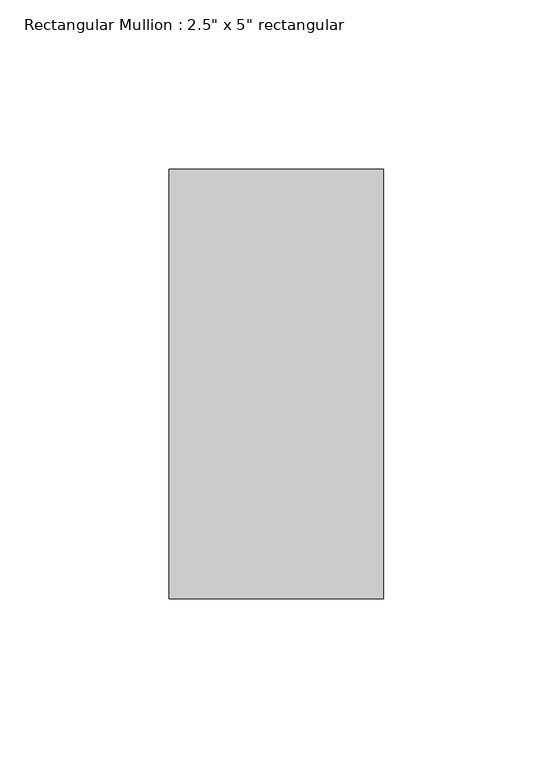
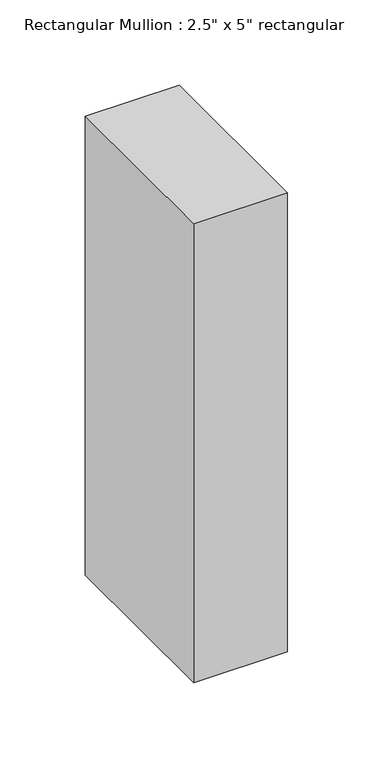
"""IFC4 building model written with IfcOpenShell, lengths in millimetres: member geometry."""

from ifc_helpers import new_model, si_unit, frame, origin, place, context, project, spatial, polyline, outline, extrude, source, transform, mapped, element, save


def member_b2f14f99(model_context):
    return source(origin(), model_context, "Body", "SweptSolid", [
        extrude(outline(polyline([(0.0, 63.5), (0.0, -63.5), (-63.5, -63.5), (-63.5, 63.5), (0.0, 63.5)])), frame((0.0, 0.0, -328.55491), z_axis=(0.0, 0.0, 1.0), x_axis=(1.0, 0.0, 0.0)), (0.0, 0.0, 1.0), 328.55491),
    ])


if __name__ == "__main__":
    model = new_model("IFC4")
    model_context = context("Model", 3, world=origin())
    ifc_project = project(units=[si_unit("LENGTHUNIT", "METRE", prefix="MILLI")], contexts=[model_context])
    site = spatial("IfcSite", under=ifc_project)
    building = spatial("IfcBuilding", under=site)
    placement = place(None, origin())
    member_shape = member_b2f14f99(model_context)
    element("IfcMember", 1, ObjectType="Rectangular Mullion : 2.5\" x 5\" rectangular", at=placement, inside=building, context=model_context, shape_type="MappedRepresentation", body=[
        mapped(member_shape, transform((0.0, 0.0, 0.0), x_axis=(1.0, 0.0, 0.0), y_axis=(0.0, 1.0, 0.0), z_axis=(0.0, 0.0, 1.0))),
    ])
    save(model, "model.ifc")

# Revit data of these elements
# Type "Rectangular Mullion : 2.5\" x 5\" rectangular"
#   built-in parameter 1007304 = 0.416667 (stored number, unit not read)
#   built-in parameter 1007301 = 0.104167 (stored number, unit not read)
#   built-in parameter 1007300 = 0.104167 (stored number, unit not read)
# Element 1 (IfcMember, "Rectangular Mullion : 2.5\" x 5\" rectangular")
#   Materials on its faces: "Aluminum"
# Materials
#   "Aluminum": class "Metal", colour RGB 247 247 247, transparency 0, Description = "Aluminum 6061", Cost = 0
